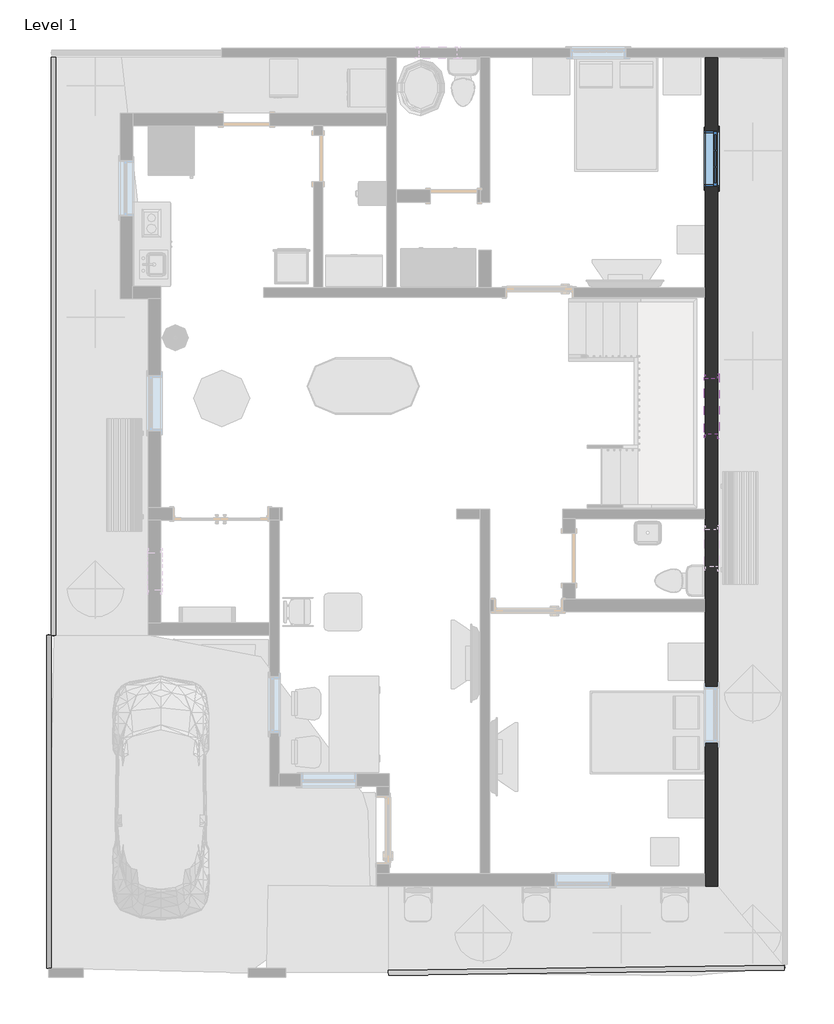
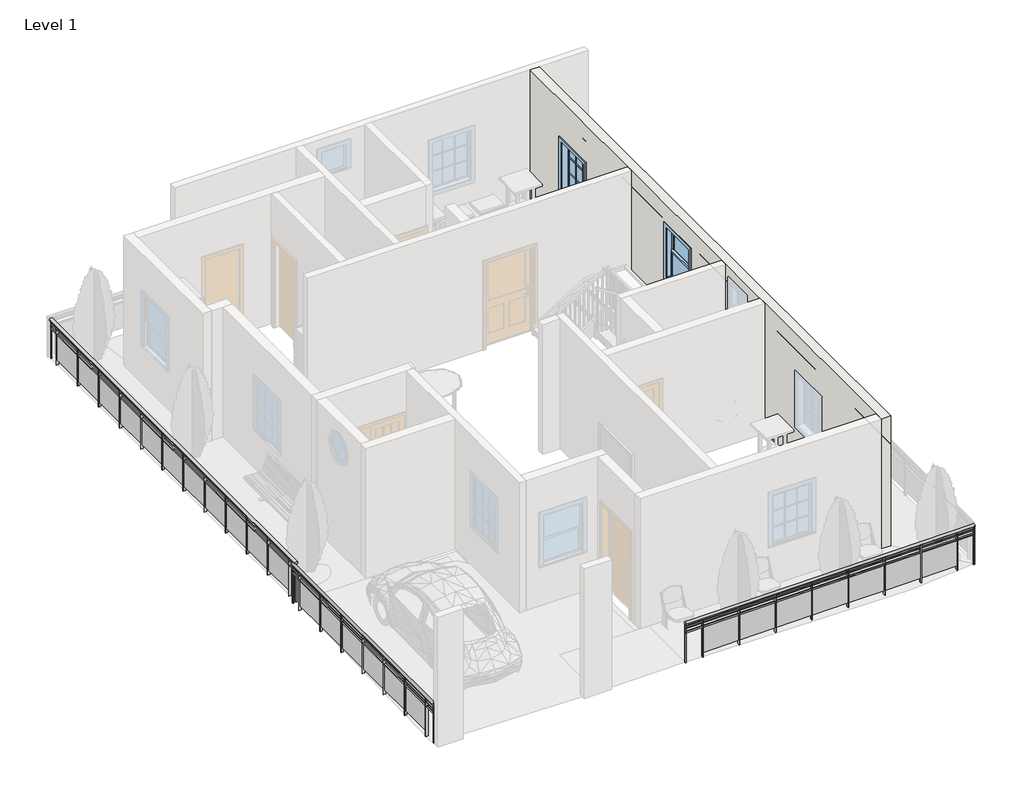
# One storey, part 2 of 4: 3 railings, 2 windows, 1 wall.
"""IFC4 building model written with IfcOpenShell, lengths in millimetres."""

from ifc_helpers import new_model, si_unit, point, frame, origin, origin_with_axes, place, context, project, spatial, polyline, ellipse_curve, trimmed, outline, extrude, faceted_brep, transform, mapped, element, save
from ifc_brep_helpers import plane_surface, extruded_surface, advanced_brep
from components import window_bd9d39db, window_31198920

model = new_model("IFC4")

# Units and contexts
model_context = context("Model", 3, world=origin())
ifc_project = project(units=[si_unit("LENGTHUNIT", "METRE", prefix="MILLI")], contexts=[model_context])

# Site, building, storey
site = spatial("IfcSite", under=ifc_project)
building = spatial("IfcBuilding", under=site)
storey = spatial("IfcBuildingStorey", under=building, Name="Level 1", Elevation=0.0)

# Railings
placement = place(None, origin())
element("IfcRailing", 1, ObjectType="Glass Panel - Bottom Fill", at=placement, inside=storey, context=model_context, shape_type="SolidModel", body=[
    advanced_brep(
    [(-5208.992213, 492.0206408, 914.4), (-5209.9447456, 568.214687, 914.4), (-11662.267213, 411.3456408, 914.4), (-11663.2197456, 487.539687, 914.4)],
    [
        (0, 1, ellipse_curve(frame((-5209.4684793, 530.1176639, 914.4), z_axis=(0.9999218666031382, 0.012500427548522056, 0.0), x_axis=(-0.012500427548522056, 0.9999218666031382, 0.0)), 38.1, 28.575)),
        (1, 0, ellipse_curve(frame((-5209.4684793, 530.1176639, 914.4), z_axis=(0.9999218666031382, 0.012500427548522056, 0.0), x_axis=(-0.012500427548522056, 0.9999218666031382, 0.0)), 38.1, 28.575)),
        (2, 3, ellipse_curve(frame((-11662.7434793, 449.4426639, 914.4), z_axis=(-0.9999218666031382, -0.012500427548522056, 0.0), x_axis=(-0.012500427548522056, 0.9999218666031382, 0.0)), 38.1, 28.575)),
        (3, 2, ellipse_curve(frame((-11662.7434793, 449.4426639, 914.4), z_axis=(-0.9999218666031382, -0.012500427548522056, 0.0), x_axis=(-0.012500427548522056, 0.9999218666031382, 0.0)), 38.1, 28.575)),
        (0, 2),
        (3, 1),
    ],
    [
        plane_surface(frame((-5209.4684793, 530.1176639, 914.4), z_axis=(0.9999218666031382, 0.012500427548522056, 0.0), x_axis=(0.012500427548522056, -0.9999218666031382, 0.0))),
        plane_surface(frame((-11662.7434793, 449.4426639, 914.4), z_axis=(-0.9999218666031382, -0.012500427548522056, 0.0), x_axis=(0.012500427548522056, -0.9999218666031382, 0.0))),
        extruded_surface(trimmed(ellipse_curve(frame((-11662.7434793, 449.4426639, 914.4), z_axis=(0.9999218666031382, 0.012500427548522056, 0.0), x_axis=(-0.012500427548522056, 0.9999218666031382, 0.0)), 38.1, 28.575), [point((-11662.267213, 411.3456408, 914.4))], [point((-11663.2197456, 487.539687, 914.4))], True, "CARTESIAN"), (6453.275, 80.67500000000001, 0.0), 6453.779255695843),
        extruded_surface(trimmed(ellipse_curve(frame((-11662.7434793, 449.4426639, 914.4), z_axis=(0.9999218666031382, 0.012500427548522056, 0.0), x_axis=(-0.012500427548522056, 0.9999218666031382, 0.0)), 38.1, 28.575), [point((-11663.2197456, 487.539687, 914.4))], [point((-11662.267213, 411.3456408, 914.4))], True, "CARTESIAN"), (6453.275, 80.67500000000001, 0.0), 6453.779255695843),
    ],
    [
        (0, [[1, 2]]),
        (1, [[3, 4]]),
        (2, [[-1, 5, -4, 6]]),
        (3, [[-2, -6, -3, -5]]),
    ],
),
    extrude(outline(polyline([(-5209.6272348, 542.8166716), (-5209.3097239, 517.4186562), (-11662.5847239, 436.7436562), (-11662.9022348, 462.1416716), (-5209.6272348, 542.8166716)])), frame((0.0, 0.0, 800.1), z_axis=(0.0, 0.0, 1.0), x_axis=(1.0, 0.0, 0.0)), (0.0, 0.0, 1.0), 25.4),
    extrude(outline(polyline([(-5209.6272348, 542.8166716), (-5209.3097239, 517.4186562), (-11662.5847239, 436.7436562), (-11662.9022348, 462.1416716), (-5209.6272348, 542.8166716)])), frame((0.0, 0.0, 698.5), z_axis=(0.0, 0.0, 1.0), x_axis=(1.0, 0.0, 0.0)), (0.0, 0.0, 1.0), 25.4),
    extrude(outline(polyline([(-11274.6517125, 479.6963407), (-11274.0166907, 428.9003099), (-11286.7156984, 428.7415545), (-11287.3507202, 479.5375853), (-11274.6517125, 479.6963407)])), origin_with_axes(), (0.0, 0.0, 1.0), 885.6788223),
    extrude(outline(polyline([(-10467.86552, 457.8446487), (-11280.6020132, 447.6843012), (-11280.6813909, 454.0338051), (-10467.9448977, 464.1941526), (-10467.86552, 457.8446487)])), frame((0.0, 0.0, 101.6), z_axis=(0.0, 0.0, 1.0), x_axis=(1.0, 0.0, 0.0)), (0.0, 0.0, 1.0), 596.9),
    extrude(outline(polyline([(-10461.9152193, 489.8566883), (-10461.2801976, 439.0606574), (-10473.9792053, 438.901902), (-10474.614227, 489.6979328), (-10461.9152193, 489.8566883)])), origin_with_axes(), (0.0, 0.0, 1.0), 885.6788223),
    extrude(outline(polyline([(-9655.1290268, 468.0049963), (-10467.86552, 457.8446487), (-10467.9448977, 464.1941526), (-9655.2084046, 474.3545001), (-9655.1290268, 468.0049963)])), frame((0.0, 0.0, 101.6), z_axis=(0.0, 0.0, 1.0), x_axis=(1.0, 0.0, 0.0)), (0.0, 0.0, 1.0), 596.9),
    extrude(outline(polyline([(-9649.1787261, 500.0170358), (-9648.5437044, 449.2210049), (-9661.2427121, 449.0622495), (-9661.8777338, 499.8582803), (-9649.1787261, 500.0170358)])), origin_with_axes(), (0.0, 0.0, 1.0), 885.6788223),
    extrude(outline(polyline([(-8842.3925337, 478.1653438), (-9655.1290268, 468.0049963), (-9655.2084046, 474.3545001), (-8842.4719114, 484.5148476), (-8842.3925337, 478.1653438)])), frame((0.0, 0.0, 101.6), z_axis=(0.0, 0.0, 1.0), x_axis=(1.0, 0.0, 0.0)), (0.0, 0.0, 1.0), 596.9),
    extrude(outline(polyline([(-8836.4422329, 510.1773833), (-8835.8072112, 459.3813525), (-8848.5062189, 459.222597), (-8849.1412406, 510.0186279), (-8836.4422329, 510.1773833)])), origin_with_axes(), (0.0, 0.0, 1.0), 885.6788223),
    extrude(outline(polyline([(-8029.6560405, 488.3256913), (-8842.3925337, 478.1653438), (-8842.4719114, 484.5148476), (-8029.7354182, 494.6751951), (-8029.6560405, 488.3256913)])), frame((0.0, 0.0, 101.6), z_axis=(0.0, 0.0, 1.0), x_axis=(1.0, 0.0, 0.0)), (0.0, 0.0, 1.0), 596.9),
    extrude(outline(polyline([(-8023.7057398, 520.3377308), (-8023.070718, 469.5417), (-8035.7697257, 469.3829445), (-8036.4047475, 520.1789754), (-8023.7057398, 520.3377308)])), origin_with_axes(), (0.0, 0.0, 1.0), 885.6788223),
    extrude(outline(polyline([(-7216.9195473, 498.4860388), (-8029.6560405, 488.3256913), (-8029.7354182, 494.6751951), (-7216.998925, 504.8355426), (-7216.9195473, 498.4860388)])), frame((0.0, 0.0, 101.6), z_axis=(0.0, 0.0, 1.0), x_axis=(1.0, 0.0, 0.0)), (0.0, 0.0, 1.0), 596.9),
    extrude(outline(polyline([(-7210.9692466, 530.4980783), (-7210.3342249, 479.7020475), (-7223.0332326, 479.5432921), (-7223.6682543, 530.3393229), (-7210.9692466, 530.4980783)])), origin_with_axes(), (0.0, 0.0, 1.0), 885.6788223),
    extrude(outline(polyline([(-6404.1830541, 508.6463863), (-7216.9195473, 498.4860388), (-7216.998925, 504.8355426), (-6404.2624319, 514.9958902), (-6404.1830541, 508.6463863)])), frame((0.0, 0.0, 101.6), z_axis=(0.0, 0.0, 1.0), x_axis=(1.0, 0.0, 0.0)), (0.0, 0.0, 1.0), 596.9),
    extrude(outline(polyline([(-6398.2327534, 540.6584258), (-6397.5977317, 489.862395), (-6410.2967394, 489.7036396), (-6410.9317611, 540.4996704), (-6398.2327534, 540.6584258)])), origin_with_axes(), (0.0, 0.0, 1.0), 885.6788223),
    extrude(outline(polyline([(-5591.446561, 518.8067338), (-6404.1830541, 508.6463863), (-6404.2624319, 514.9958902), (-5591.5259387, 525.1562377), (-5591.446561, 518.8067338)])), frame((0.0, 0.0, 101.6), z_axis=(0.0, 0.0, 1.0), x_axis=(1.0, 0.0, 0.0)), (0.0, 0.0, 1.0), 596.9),
    extrude(outline(polyline([(-5585.4962602, 550.8187733), (-5584.8612385, 500.0227425), (-5597.5602462, 499.8639871), (-5598.1952679, 550.6600179), (-5585.4962602, 550.8187733)])), origin_with_axes(), (0.0, 0.0, 1.0), 885.6788223),
    extrude(outline(polyline([(-11650.1635382, 459.1256751), (-11649.9254051, 440.0771636), (-11668.9739166, 439.8390304), (-11669.2120498, 458.887542), (-11650.1635382, 459.1256751)])), origin_with_axes(), (0.0, 0.0, 1.0), 885.6788223),
    extrude(outline(polyline([(-5203.2380421, 539.7212974), (-5202.9999089, 520.6727858), (-5222.0484205, 520.4346527), (-5222.2865536, 539.4831643), (-5203.2380421, 539.7212974)])), origin_with_axes(), (0.0, 0.0, 1.0), 885.6788223),
])
element("IfcRailing", 2, ObjectType="Glass Panel - Bottom Fill", at=placement, inside=storey, context=model_context, shape_type="SolidModel", body=[
    advanced_brep(
    [(-17161.8434793, 5952.1610583, 914.4), (-17085.6434793, 5952.1610583, 914.4), (-17161.8434793, 15373.2426639, 914.4), (-17085.6434793, 15373.2426639, 914.4)],
    [
        (0, 1, ellipse_curve(frame((-17123.7434793, 5952.1610583, 914.4), z_axis=(0.0, -1.0, 0.0), x_axis=(1.0, 0.0, 0.0)), 38.1, 28.575)),
        (1, 0, ellipse_curve(frame((-17123.7434793, 5952.1610583, 914.4), z_axis=(0.0, -1.0, 0.0), x_axis=(1.0, 0.0, 0.0)), 38.1, 28.575)),
        (2, 3, ellipse_curve(frame((-17123.7434793, 15373.2426639, 914.4), z_axis=(0.0, 1.0, 0.0), x_axis=(1.0, 0.0, 0.0)), 38.1, 28.575)),
        (3, 2, ellipse_curve(frame((-17123.7434793, 15373.2426639, 914.4), z_axis=(0.0, 1.0, 0.0), x_axis=(1.0, 0.0, 0.0)), 38.1, 28.575)),
        (0, 2),
        (3, 1),
    ],
    [
        plane_surface(frame((-17123.7434793, 5952.1610583, 914.4), z_axis=(0.0, -1.0, 0.0), x_axis=(0.0, 0.0, 1.0))),
        plane_surface(frame((-17123.7434793, 15373.2426639, 914.4), z_axis=(0.0, 1.0, 0.0), x_axis=(0.0, 0.0, 1.0))),
        extruded_surface(trimmed(ellipse_curve(frame((-17123.7434793, 15373.2426639, 914.4), z_axis=(0.0, -1.0, 0.0), x_axis=(1.0, 0.0, 0.0)), 38.1, 28.575), [point((-17161.8434793, 15373.2426639, 914.4))], [point((-17085.6434793, 15373.2426639, 914.4))], True, "CARTESIAN"), (0.0, -9421.0816056, 0.0), 9421.0816056),
        extruded_surface(trimmed(ellipse_curve(frame((-17123.7434793, 15373.2426639, 914.4), z_axis=(0.0, -1.0, 0.0), x_axis=(1.0, 0.0, 0.0)), 38.1, 28.575), [point((-17085.6434793, 15373.2426639, 914.4))], [point((-17161.8434793, 15373.2426639, 914.4))], True, "CARTESIAN"), (0.0, -9421.0816056, 0.0), 9421.0816056),
    ],
    [
        (0, [[1, 2]]),
        (1, [[3, 4]]),
        (2, [[-1, 5, -4, 6]]),
        (3, [[-2, -6, -3, -5]]),
    ],
),
    extrude(outline(polyline([(-17111.0434793, 5952.1610583), (-17136.4434793, 5952.1610583), (-17136.4434793, 15373.2426639), (-17111.0434793, 15373.2426639), (-17111.0434793, 5952.1610583)])), frame((0.0, 0.0, 800.1), z_axis=(0.0, 0.0, 1.0), x_axis=(1.0, 0.0, 0.0)), (0.0, 0.0, 1.0), 25.4),
    extrude(outline(polyline([(-17111.0434793, 5952.1610583), (-17136.4434793, 5952.1610583), (-17136.4434793, 15373.2426639), (-17111.0434793, 15373.2426639), (-17111.0434793, 5952.1610583)])), frame((0.0, 0.0, 698.5), z_axis=(0.0, 0.0, 1.0), x_axis=(1.0, 0.0, 0.0)), (0.0, 0.0, 1.0), 25.4),
    extrude(outline(polyline([(-17098.3434793, 15126.7518611), (-17149.1434793, 15126.7518611), (-17149.1434793, 15139.4518611), (-17098.3434793, 15139.4518611), (-17098.3434793, 15126.7518611)])), origin_with_axes(), (0.0, 0.0, 1.0), 885.6788223),
    extrude(outline(polyline([(-17130.2786363, 14320.3018611), (-17130.2786363, 15133.1018611), (-17123.9286363, 15133.1018611), (-17123.9286363, 14320.3018611), (-17130.2786363, 14320.3018611)])), frame((0.0, 0.0, 101.6), z_axis=(0.0, 0.0, 1.0), x_axis=(1.0, 0.0, 0.0)), (0.0, 0.0, 1.0), 596.9),
    extrude(outline(polyline([(-17098.3434793, 14313.9518611), (-17149.1434793, 14313.9518611), (-17149.1434793, 14326.6518611), (-17098.3434793, 14326.6518611), (-17098.3434793, 14313.9518611)])), origin_with_axes(), (0.0, 0.0, 1.0), 885.6788223),
    extrude(outline(polyline([(-17130.2786363, 13507.5018611), (-17130.2786363, 14320.3018611), (-17123.9286363, 14320.3018611), (-17123.9286363, 13507.5018611), (-17130.2786363, 13507.5018611)])), frame((0.0, 0.0, 101.6), z_axis=(0.0, 0.0, 1.0), x_axis=(1.0, 0.0, 0.0)), (0.0, 0.0, 1.0), 596.9),
    extrude(outline(polyline([(-17098.3434793, 13501.1518611), (-17149.1434793, 13501.1518611), (-17149.1434793, 13513.8518611), (-17098.3434793, 13513.8518611), (-17098.3434793, 13501.1518611)])), origin_with_axes(), (0.0, 0.0, 1.0), 885.6788223),
    extrude(outline(polyline([(-17130.2786363, 12694.7018611), (-17130.2786363, 13507.5018611), (-17123.9286363, 13507.5018611), (-17123.9286363, 12694.7018611), (-17130.2786363, 12694.7018611)])), frame((0.0, 0.0, 101.6), z_axis=(0.0, 0.0, 1.0), x_axis=(1.0, 0.0, 0.0)), (0.0, 0.0, 1.0), 596.9),
    extrude(outline(polyline([(-17098.3434793, 12688.3518611), (-17149.1434793, 12688.3518611), (-17149.1434793, 12701.0518611), (-17098.3434793, 12701.0518611), (-17098.3434793, 12688.3518611)])), origin_with_axes(), (0.0, 0.0, 1.0), 885.6788223),
    extrude(outline(polyline([(-17130.2786363, 11881.9018611), (-17130.2786363, 12694.7018611), (-17123.9286363, 12694.7018611), (-17123.9286363, 11881.9018611), (-17130.2786363, 11881.9018611)])), frame((0.0, 0.0, 101.6), z_axis=(0.0, 0.0, 1.0), x_axis=(1.0, 0.0, 0.0)), (0.0, 0.0, 1.0), 596.9),
    extrude(outline(polyline([(-17098.3434793, 11875.5518611), (-17149.1434793, 11875.5518611), (-17149.1434793, 11888.2518611), (-17098.3434793, 11888.2518611), (-17098.3434793, 11875.5518611)])), origin_with_axes(), (0.0, 0.0, 1.0), 885.6788223),
    extrude(outline(polyline([(-17130.2786363, 11069.1018611), (-17130.2786363, 11881.9018611), (-17123.9286363, 11881.9018611), (-17123.9286363, 11069.1018611), (-17130.2786363, 11069.1018611)])), frame((0.0, 0.0, 101.6), z_axis=(0.0, 0.0, 1.0), x_axis=(1.0, 0.0, 0.0)), (0.0, 0.0, 1.0), 596.9),
    extrude(outline(polyline([(-17098.3434793, 11062.7518611), (-17149.1434793, 11062.7518611), (-17149.1434793, 11075.4518611), (-17098.3434793, 11075.4518611), (-17098.3434793, 11062.7518611)])), origin_with_axes(), (0.0, 0.0, 1.0), 885.6788223),
    extrude(outline(polyline([(-17130.2786363, 10256.3018611), (-17130.2786363, 11069.1018611), (-17123.9286363, 11069.1018611), (-17123.9286363, 10256.3018611), (-17130.2786363, 10256.3018611)])), frame((0.0, 0.0, 101.6), z_axis=(0.0, 0.0, 1.0), x_axis=(1.0, 0.0, 0.0)), (0.0, 0.0, 1.0), 596.9),
    extrude(outline(polyline([(-17098.3434793, 10249.9518611), (-17149.1434793, 10249.9518611), (-17149.1434793, 10262.6518611), (-17098.3434793, 10262.6518611), (-17098.3434793, 10249.9518611)])), origin_with_axes(), (0.0, 0.0, 1.0), 885.6788223),
    extrude(outline(polyline([(-17130.2786363, 9443.5018611), (-17130.2786363, 10256.3018611), (-17123.9286363, 10256.3018611), (-17123.9286363, 9443.5018611), (-17130.2786363, 9443.5018611)])), frame((0.0, 0.0, 101.6), z_axis=(0.0, 0.0, 1.0), x_axis=(1.0, 0.0, 0.0)), (0.0, 0.0, 1.0), 596.9),
    extrude(outline(polyline([(-17098.3434793, 9437.1518611), (-17149.1434793, 9437.1518611), (-17149.1434793, 9449.8518611), (-17098.3434793, 9449.8518611), (-17098.3434793, 9437.1518611)])), origin_with_axes(), (0.0, 0.0, 1.0), 885.6788223),
    extrude(outline(polyline([(-17130.2786363, 8630.7018611), (-17130.2786363, 9443.5018611), (-17123.9286363, 9443.5018611), (-17123.9286363, 8630.7018611), (-17130.2786363, 8630.7018611)])), frame((0.0, 0.0, 101.6), z_axis=(0.0, 0.0, 1.0), x_axis=(1.0, 0.0, 0.0)), (0.0, 0.0, 1.0), 596.9),
    extrude(outline(polyline([(-17098.3434793, 8624.3518611), (-17149.1434793, 8624.3518611), (-17149.1434793, 8637.0518611), (-17098.3434793, 8637.0518611), (-17098.3434793, 8624.3518611)])), origin_with_axes(), (0.0, 0.0, 1.0), 885.6788223),
    extrude(outline(polyline([(-17130.2786363, 7817.9018611), (-17130.2786363, 8630.7018611), (-17123.9286363, 8630.7018611), (-17123.9286363, 7817.9018611), (-17130.2786363, 7817.9018611)])), frame((0.0, 0.0, 101.6), z_axis=(0.0, 0.0, 1.0), x_axis=(1.0, 0.0, 0.0)), (0.0, 0.0, 1.0), 596.9),
    extrude(outline(polyline([(-17098.3434793, 7811.5518611), (-17149.1434793, 7811.5518611), (-17149.1434793, 7824.2518611), (-17098.3434793, 7824.2518611), (-17098.3434793, 7811.5518611)])), origin_with_axes(), (0.0, 0.0, 1.0), 885.6788223),
    extrude(outline(polyline([(-17130.2786363, 7005.1018611), (-17130.2786363, 7817.9018611), (-17123.9286363, 7817.9018611), (-17123.9286363, 7005.1018611), (-17130.2786363, 7005.1018611)])), frame((0.0, 0.0, 101.6), z_axis=(0.0, 0.0, 1.0), x_axis=(1.0, 0.0, 0.0)), (0.0, 0.0, 1.0), 596.9),
    extrude(outline(polyline([(-17098.3434793, 6998.7518611), (-17149.1434793, 6998.7518611), (-17149.1434793, 7011.4518611), (-17098.3434793, 7011.4518611), (-17098.3434793, 6998.7518611)])), origin_with_axes(), (0.0, 0.0, 1.0), 885.6788223),
    extrude(outline(polyline([(-17130.2786363, 6192.3018611), (-17130.2786363, 7005.1018611), (-17123.9286363, 7005.1018611), (-17123.9286363, 6192.3018611), (-17130.2786363, 6192.3018611)])), frame((0.0, 0.0, 101.6), z_axis=(0.0, 0.0, 1.0), x_axis=(1.0, 0.0, 0.0)), (0.0, 0.0, 1.0), 596.9),
    extrude(outline(polyline([(-17098.3434793, 6185.9518611), (-17149.1434793, 6185.9518611), (-17149.1434793, 6198.6518611), (-17098.3434793, 6198.6518611), (-17098.3434793, 6185.9518611)])), origin_with_axes(), (0.0, 0.0, 1.0), 885.6788223),
    extrude(outline(polyline([(-17114.2184793, 15360.5426639), (-17133.2684793, 15360.5426639), (-17133.2684793, 15379.5926639), (-17114.2184793, 15379.5926639), (-17114.2184793, 15360.5426639)])), origin_with_axes(), (0.0, 0.0, 1.0), 885.6788223),
    extrude(outline(polyline([(-17114.2184793, 5945.8110583), (-17133.2684793, 5945.8110583), (-17133.2684793, 5964.8610583), (-17114.2184793, 5964.8610583), (-17114.2184793, 5945.8110583)])), origin_with_axes(), (0.0, 0.0, 1.0), 885.6788223),
])
element("IfcRailing", 3, ObjectType="Glass Panel - Bottom Fill", at=placement, inside=storey, context=model_context, shape_type="SolidModel", body=[
    advanced_brep(
    [(-17161.8434793, 5952.1610583, 914.4), (-17238.0434793, 5952.1610583, 914.4), (-17161.8434793, 525.6426639, 914.4), (-17238.0434793, 525.6426639, 914.4)],
    [
        (0, 1, ellipse_curve(frame((-17199.9434793, 5952.1610583, 914.4), z_axis=(0.0, 1.0, 0.0), x_axis=(-1.0, 0.0, 0.0)), 38.1, 28.575)),
        (1, 0, ellipse_curve(frame((-17199.9434793, 5952.1610583, 914.4), z_axis=(0.0, 1.0, 0.0), x_axis=(-1.0, 0.0, 0.0)), 38.1, 28.575)),
        (2, 3, ellipse_curve(frame((-17199.9434793, 525.6426639, 914.4), z_axis=(0.0, -1.0, 0.0), x_axis=(-1.0, 0.0, 0.0)), 38.1, 28.575)),
        (3, 2, ellipse_curve(frame((-17199.9434793, 525.6426639, 914.4), z_axis=(0.0, -1.0, 0.0), x_axis=(-1.0, 0.0, 0.0)), 38.1, 28.575)),
        (0, 2),
        (3, 1),
    ],
    [
        plane_surface(frame((-17199.9434793, 5952.1610583, 914.4), z_axis=(0.0, 1.0, 0.0), x_axis=(0.0, 0.0, -1.0))),
        plane_surface(frame((-17199.9434793, 525.6426639, 914.4), z_axis=(0.0, -1.0, 0.0), x_axis=(0.0, 0.0, -1.0))),
        extruded_surface(trimmed(ellipse_curve(frame((-17199.9434793, 525.6426639, 914.4), z_axis=(0.0, 1.0, 0.0), x_axis=(-1.0, 0.0, 0.0)), 38.1, 28.575), [point((-17161.8434793, 525.6426639, 914.4))], [point((-17238.0434793, 525.6426639, 914.4))], True, "CARTESIAN"), (0.0, 5426.5183944, 0.0), 5426.5183944),
        extruded_surface(trimmed(ellipse_curve(frame((-17199.9434793, 525.6426639, 914.4), z_axis=(0.0, 1.0, 0.0), x_axis=(-1.0, 0.0, 0.0)), 38.1, 28.575), [point((-17238.0434793, 525.6426639, 914.4))], [point((-17161.8434793, 525.6426639, 914.4))], True, "CARTESIAN"), (0.0, 5426.5183944, 0.0), 5426.5183944),
    ],
    [
        (0, [[1, 2]]),
        (1, [[3, 4]]),
        (2, [[-1, 5, -4, 6]]),
        (3, [[-2, -6, -3, -5]]),
    ],
),
    extrude(outline(polyline([(-17212.6434793, 5952.1610583), (-17187.2434793, 5952.1610583), (-17187.2434793, 525.6426639), (-17212.6434793, 525.6426639), (-17212.6434793, 5952.1610583)])), frame((0.0, 0.0, 800.1), z_axis=(0.0, 0.0, 1.0), x_axis=(1.0, 0.0, 0.0)), (0.0, 0.0, 1.0), 25.4),
    extrude(outline(polyline([(-17212.6434793, 5952.1610583), (-17187.2434793, 5952.1610583), (-17187.2434793, 525.6426639), (-17212.6434793, 525.6426639), (-17212.6434793, 5952.1610583)])), frame((0.0, 0.0, 698.5), z_axis=(0.0, 0.0, 1.0), x_axis=(1.0, 0.0, 0.0)), (0.0, 0.0, 1.0), 25.4),
    extrude(outline(polyline([(-17225.3434793, 806.8518611), (-17174.5434793, 806.8518611), (-17174.5434793, 794.1518611), (-17225.3434793, 794.1518611), (-17225.3434793, 806.8518611)])), origin_with_axes(), (0.0, 0.0, 1.0), 885.6788223),
    extrude(outline(polyline([(-17193.4083223, 1613.3018611), (-17193.4083223, 800.5018611), (-17199.7583223, 800.5018611), (-17199.7583223, 1613.3018611), (-17193.4083223, 1613.3018611)])), frame((0.0, 0.0, 101.6), z_axis=(0.0, 0.0, 1.0), x_axis=(1.0, 0.0, 0.0)), (0.0, 0.0, 1.0), 596.9),
    extrude(outline(polyline([(-17225.3434793, 1619.6518611), (-17174.5434793, 1619.6518611), (-17174.5434793, 1606.9518611), (-17225.3434793, 1606.9518611), (-17225.3434793, 1619.6518611)])), origin_with_axes(), (0.0, 0.0, 1.0), 885.6788223),
    extrude(outline(polyline([(-17193.4083223, 2426.1018611), (-17193.4083223, 1613.3018611), (-17199.7583223, 1613.3018611), (-17199.7583223, 2426.1018611), (-17193.4083223, 2426.1018611)])), frame((0.0, 0.0, 101.6), z_axis=(0.0, 0.0, 1.0), x_axis=(1.0, 0.0, 0.0)), (0.0, 0.0, 1.0), 596.9),
    extrude(outline(polyline([(-17225.3434793, 2432.4518611), (-17174.5434793, 2432.4518611), (-17174.5434793, 2419.7518611), (-17225.3434793, 2419.7518611), (-17225.3434793, 2432.4518611)])), origin_with_axes(), (0.0, 0.0, 1.0), 885.6788223),
    extrude(outline(polyline([(-17193.4083223, 3238.9018611), (-17193.4083223, 2426.1018611), (-17199.7583223, 2426.1018611), (-17199.7583223, 3238.9018611), (-17193.4083223, 3238.9018611)])), frame((0.0, 0.0, 101.6), z_axis=(0.0, 0.0, 1.0), x_axis=(1.0, 0.0, 0.0)), (0.0, 0.0, 1.0), 596.9),
    extrude(outline(polyline([(-17225.3434793, 3245.2518611), (-17174.5434793, 3245.2518611), (-17174.5434793, 3232.5518611), (-17225.3434793, 3232.5518611), (-17225.3434793, 3245.2518611)])), origin_with_axes(), (0.0, 0.0, 1.0), 885.6788223),
    extrude(outline(polyline([(-17193.4083223, 4051.7018611), (-17193.4083223, 3238.9018611), (-17199.7583223, 3238.9018611), (-17199.7583223, 4051.7018611), (-17193.4083223, 4051.7018611)])), frame((0.0, 0.0, 101.6), z_axis=(0.0, 0.0, 1.0), x_axis=(1.0, 0.0, 0.0)), (0.0, 0.0, 1.0), 596.9),
    extrude(outline(polyline([(-17225.3434793, 4058.0518611), (-17174.5434793, 4058.0518611), (-17174.5434793, 4045.3518611), (-17225.3434793, 4045.3518611), (-17225.3434793, 4058.0518611)])), origin_with_axes(), (0.0, 0.0, 1.0), 885.6788223),
    extrude(outline(polyline([(-17193.4083223, 4864.5018611), (-17193.4083223, 4051.7018611), (-17199.7583223, 4051.7018611), (-17199.7583223, 4864.5018611), (-17193.4083223, 4864.5018611)])), frame((0.0, 0.0, 101.6), z_axis=(0.0, 0.0, 1.0), x_axis=(1.0, 0.0, 0.0)), (0.0, 0.0, 1.0), 596.9),
    extrude(outline(polyline([(-17225.3434793, 4870.8518611), (-17174.5434793, 4870.8518611), (-17174.5434793, 4858.1518611), (-17225.3434793, 4858.1518611), (-17225.3434793, 4870.8518611)])), origin_with_axes(), (0.0, 0.0, 1.0), 885.6788223),
    extrude(outline(polyline([(-17193.4083223, 5677.3018611), (-17193.4083223, 4864.5018611), (-17199.7583223, 4864.5018611), (-17199.7583223, 5677.3018611), (-17193.4083223, 5677.3018611)])), frame((0.0, 0.0, 101.6), z_axis=(0.0, 0.0, 1.0), x_axis=(1.0, 0.0, 0.0)), (0.0, 0.0, 1.0), 596.9),
    extrude(outline(polyline([(-17225.3434793, 5683.6518611), (-17174.5434793, 5683.6518611), (-17174.5434793, 5670.9518611), (-17225.3434793, 5670.9518611), (-17225.3434793, 5683.6518611)])), origin_with_axes(), (0.0, 0.0, 1.0), 885.6788223),
    extrude(outline(polyline([(-17209.4684793, 538.3426639), (-17190.4184793, 538.3426639), (-17190.4184793, 519.2926639), (-17209.4684793, 519.2926639), (-17209.4684793, 538.3426639)])), origin_with_axes(), (0.0, 0.0, 1.0), 885.6788223),
    extrude(outline(polyline([(-17209.4684793, 5958.5110583), (-17190.4184793, 5958.5110583), (-17190.4184793, 5939.4610583), (-17209.4684793, 5939.4610583), (-17209.4684793, 5958.5110583)])), origin_with_axes(), (0.0, 0.0, 1.0), 885.6788223),
])

# Wall
element("IfcWall", 4, ObjectType="Generic - 8\"", at=placement, inside=storey, context=model_context, shape_type="Brep", body=[
    faceted_brep([(-6495.3434793, 15373.2426639, 0.0), (-6495.3434793, 11616.3610583, 0.0), (-6495.3434793, 11463.9610583, 0.0), (-6495.3434793, 8007.2426639, 0.0), (-6495.3434793, 7854.8426639, 0.0), (-6495.3434793, 6536.3610583, 0.0), (-6495.3434793, 6333.1610583, 0.0), (-6495.3434793, 2063.6426639, 0.0), (-6495.3434793, 1860.4426639, 0.0), (-6495.3434793, 1860.4426639, 3048.0), (-6495.3434793, 2063.6426639, 3048.0), (-6495.3434793, 6333.1610583, 3048.0), (-6495.3434793, 6536.3610583, 3048.0), (-6495.3434793, 7854.8426639, 3048.0), (-6495.3434793, 8007.2426639, 3048.0), (-6495.3434793, 11463.9610583, 3048.0), (-6495.3434793, 11616.3610583, 3048.0), (-6495.3434793, 15373.2426639, 3048.0), (-6495.3434793, 4199.5610583, 2133.6), (-6495.3434793, 4199.5610583, 914.4), (-6495.3434793, 5113.9610583, 914.4), (-6495.3434793, 5113.9610583, 2133.6), (-6495.3434793, 13265.0426639, 2133.6), (-6495.3434793, 13265.0426639, 914.4), (-6495.3434793, 14179.4426639, 914.4), (-6495.3434793, 14179.4426639, 2133.6), (-6495.3434793, 9228.7610583, 2565.4), (-6495.3434793, 9228.7610583, 1346.2), (-6495.3434793, 10143.1610583, 1346.2), (-6495.3434793, 10143.1610583, 2565.4), (-6495.3434793, 7067.4426639, 2768.6), (-6495.3434793, 7067.4426639, 2159.0), (-6495.3434793, 7677.0426639, 2159.0), (-6495.3434793, 7677.0426639, 2768.6), (-6292.1434793, 15373.2426639, 0.0), (-6292.1434793, 15373.2426639, 3048.0), (-6292.1434793, 1860.4426639, 3048.0), (-6292.1434793, 1860.4426639, 0.0), (-6292.1434793, 4199.5610583, 2133.6), (-6292.1434793, 5113.9610583, 2133.6), (-6292.1434793, 5113.9610583, 914.4), (-6292.1434793, 4199.5610583, 914.4), (-6292.1434793, 13265.0426639, 2133.6), (-6292.1434793, 14179.4426639, 2133.6), (-6292.1434793, 14179.4426639, 914.4), (-6292.1434793, 13265.0426639, 914.4), (-6292.1434793, 9228.7610583, 2565.4), (-6292.1434793, 10143.1610583, 2565.4), (-6292.1434793, 10143.1610583, 1346.2), (-6292.1434793, 9228.7610583, 1346.2), (-6292.1434793, 7067.4426639, 2768.6), (-6292.1434793, 7677.0426639, 2768.6), (-6292.1434793, 7677.0426639, 2159.0), (-6292.1434793, 7067.4426639, 2159.0)], [[[0, 1, 2, 3, 4, 5, 6, 7, 8, 9, 10, 11, 12, 13, 14, 15, 16, 17], [18, 19, 20, 21], [22, 23, 24, 25], [26, 27, 28, 29], [30, 31, 32, 33]], [[34, 35, 36, 37], [38, 39, 40, 41], [42, 43, 44, 45], [46, 47, 48, 49], [50, 51, 52, 53]], [[8, 7, 6, 5, 4, 3, 2, 1, 0, 34, 37]], [[17, 16, 15, 14, 13, 12, 11, 10, 9, 36, 35]], [[0, 17, 35, 34]], [[9, 8, 37, 36]], [[19, 18, 38, 41]], [[20, 19, 41, 40]], [[21, 20, 40, 39]], [[18, 21, 39, 38]], [[23, 22, 42, 45]], [[24, 23, 45, 44]], [[25, 24, 44, 43]], [[22, 25, 43, 42]], [[27, 26, 46, 49]], [[28, 27, 49, 48]], [[29, 28, 48, 47]], [[26, 29, 47, 46]], [[31, 30, 50, 53]], [[32, 31, 53, 52]], [[33, 32, 52, 51]], [[30, 33, 51, 50]]]),
])

# Windows
window_shape = window_bd9d39db(model_context)
element("IfcWindow", 5, ObjectType="Casement 3x3 with Trim : 36\" x 48\"", at=placement, inside=storey, context=model_context, shape_type="MappedRepresentation", body=[
    mapped(window_shape, transform((-6393.7434793, 13722.2426639, -304.8), x_axis=(0.0, -1.0, 0.0), y_axis=(1.0, 0.0, 0.0), z_axis=(0.0, 0.0, 1.0))),
])
window_2_shape = window_31198920(model_context)
element("IfcWindow", 6, ObjectType="Double Hung with Trim : 36\" x 48\"", at=placement, inside=storey, context=model_context, shape_type="MappedRepresentation", body=[
    mapped(window_2_shape, transform((-6393.7434793, 9685.9610583, 431.8), x_axis=(0.0, -1.0, 0.0), y_axis=(1.0, 0.0, 0.0), z_axis=(0.0, 0.0, 1.0))),
])

save(model, "model.ifc")

# Revit data of these elements
# Type "Glass Panel - Bottom Fill"
#   Assembly Code = "C2010400"
#   built-in parameter 1008612 = 0.0416667 (stored number, unit not read)
#   built-in parameter 1008611 = 0.0416667 (stored number, unit not read)
#   built-in parameter 1008609 = 0.333333 (stored number, unit not read)
#   built-in parameter 1008604 = 0.166667 (stored number, unit not read)
#   built-in parameter 1008603 = 0.166667 (stored number, unit not read)
#   Railing Height = 3' - 0"
#   built-in parameter 1008630 = 2
#   built-in parameter 1008610 = 2
#   built-in parameter 1008618 = Baluster - Square : 3/4"
# Type "Generic - 8\""
#   Assembly Code = "B2010"
#   Layers, outside or top first: 0' - 8" "Brick, Common" (function 1)
# Type "Casement 3x3 with Trim : 36\" x 48\""
#   Type Mark = "10"
#   Construction Type Id = "GSP4R"
#   Assembly Code = "B2020100"
#   Analytic Construction = "1/8 in Pilkington single glazing"
#   Visual Light Transmittance = 0.9
#   Solar Heat Gain Coefficient = 0.78
#   Heat Transfer Coefficient (U) = 0.6496 BTU/(h·ft²·°F)
#   Height = 4' - 0"
#   Default Sill Height = 4' - 0"
#   Trim Projection - Ext. = 0' - 0 1/2"
#   Trim Projection - Int. = 0' - 0 3/4"
#   Trim Width - Exterior = 0' - 3 1/2"
#   Trim Width - Interior = 0' - 3 1/2"
#   Width = 3' - 0"
#   Window Inset = 0' - 0 3/4"
#   Define Thermal Properties by = 1
#   Glass Pane Material = Glass
#   Sash Material = Sash
#   Trim Exterior Material = Trim
#   Trim Interior Material = Trim
#   Wall Closure = (empty or 0)
# Type "Double Hung with Trim : 36\" x 48\""
#   Type Mark = "13"
#   Construction Type Id = "GSP4R"
#   Assembly Code = "B2020100"
#   Analytic Construction = "1/8 in Pilkington single glazing"
#   Visual Light Transmittance = 0.9
#   Solar Heat Gain Coefficient = 0.78
#   Heat Transfer Coefficient (U) = 0.6496 BTU/(h·ft²·°F)
#   Height = 4' - 0"
#   Default Sill Height = 3' - 0"
#   Trim Projection - Ext. = 0' - 0 1/2"
#   Trim Projection - Int. = 0' - 0 3/4"
#   Trim Width - Exterior = 0' - 3 1/2"
#   Trim Width - Interior = 0' - 3 1/2"
#   Width = 3' - 0"
#   Window Inset = 0' - 0 3/4"
#   Define Thermal Properties by = 1
#   Glass Pane Material = Glass
#   Sash Material = Sash
#   Trim Exterior Material = Trim
#   Trim Interior Material = Trim
#   Wall Closure = (empty or 0)
# Elements 1, 2, 3 (IfcRailing, "Glass Panel - Bottom Fill")
#   Phase Created = New Construction
#   Materials on its faces: "Glass"
# Element 4 (IfcWall, "Generic - 8\"")
#   Top Offset = 0' - 0"
#   Base Offset = 0' - 0"
#   Unconnected Height = 10' - 0"
#   wall height = 10' - 0"
#   Phase Created = New Construction
#   Base Constraint = Level 1
#   Materials on its faces: "Brick, Common"
# Element 5 (IfcWindow, "Casement 3x3 with Trim : 36\" x 48\"")
#   Mark = "4"
#   Phase Created = New Construction
#   Materials on its faces: "Sash", "Glass", "Trim"
# Element 6 (IfcWindow, "Double Hung with Trim : 36\" x 48\"")
#   Mark = "10"
#   Phase Created = New Construction
#   Materials on its faces: "Sash", "Trim", "Glass"
# Materials
#   "Brick, Common": class "Masonry", colour RGB 170 98 104, transparency 0, Description = "Common brick", Cost = 0
#   "Glass": class "Glass", colour RGB 0 128 192, transparency 0.75, Description = "Soda Lime Glass", Cost = 0
#   "Sash": class "Wood", colour RGB 224 178 126, transparency 0
#   "Trim": class "Wood", colour RGB 224 178 126, transparency 0
